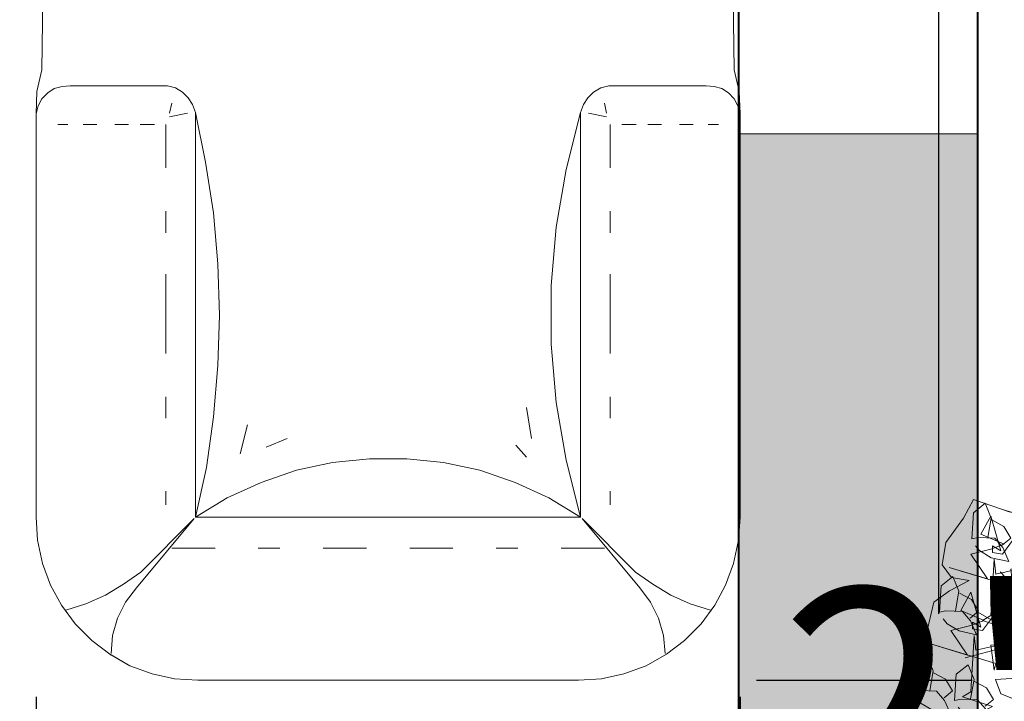
# Model space of a CAD drawing. Units: inches. Extents: x 2337 to 3570, y 1258 to 1938.
# Tile 10 of 30: x 2837 to 2874, y 1626 to 1651. Entities that reach past the tile are written whole.
import ezdxf

# ---------------------------------------------------------------- set-up
doc = ezdxf.new("R2010")
doc.units = ezdxf.units.IN
for name, color, linetype, lineweight in [('A-ANNO-DIMS', 2, 'Continuous', 18), ('A-GLAZ', 4, 'Continuous', 18), ('A-WALL', 7, 'Continuous', 40), ('ARBOL', 74, 'Continuous', 13), ('furn', 8, 'Continuous', 18)]:
    doc.layers.add(name, color=color, linetype=linetype, lineweight=lineweight)
doc.layers.add('A-WALL-PATT', color=18, linetype='Continuous', lineweight=13, true_color=0x000000)
doc.styles.get("Standard").update_dxf_attribs({"font": 'arial.ttf'})
doc.dimstyles.new('ISO-25', dxfattribs={"dimtxt": 9, "dimasz": 2.5, "dimexe": 1.25, "dimexo": 0.625, "dimtad": 1, "dimdec": 1, "dimlunit": 3, "dimtxsty": 'Standard', "dimcen": 2.5, "dimadec": 0, "dimazin": 0, "dimtfac": 1, "dimtdec": 1, "dimtmove": 0, "dimatfit": 3, "dimfxl": 1, "dimarcsym": 0})

# ---------------------------------------------------------------- blocks, each defined once
blk = doc.blocks.new('sofa-49')
at = {"color": 0, "linetype": 'ByBlock'}
for p, q in [((-0.1827, 1.5875), (-0.1944, 0.7614)), ((-0.1827, 1.5875), (-0.1944, 0.7614)), ((0.6696, 0.7614), (0.6579, 1.5875)), ((0.6696, 0.7614), (0.6579, 1.5875)), ((-0.1944, 0.7614), (-0.2007, 0.7344)), ((-0.1944, 0.7614), (-0.2007, 0.7344)), ((0.6759, 0.7344), (0.6696, 0.7614)), ((0.6759, 0.7344), (0.6696, 0.7614)), ((-0.1872, 0.7326), (-0.1791, 0.738)), ((-0.1791, 0.738), (-0.1692, 0.7407)), ((-0.1692, 0.7407), (-0.1593, 0.7416)), ((-0.1593, 0.7416), (-0.0486, 0.7416)), ((-0.0486, 0.7416), (-0.0378, 0.7416)), ((-0.0378, 0.7416), (-0.0279, 0.7389)), ((-0.0279, 0.7389), (-0.0189, 0.7335)), ((0.4941, 0.7335), (0.5031, 0.7389)), ((0.5031, 0.7389), (0.513, 0.7416)), ((0.513, 0.7416), (0.5238, 0.7416)), ((0.5238, 0.7416), (0.6345, 0.7416)), ((0.6345, 0.7416), (0.6444, 0.7407)), ((0.6444, 0.7407), (0.6543, 0.738)), ((0.6543, 0.738), (0.6624, 0.7326)), ((-0.2007, 0.7344), (-0.2016, 0.7065)), ((-0.2007, 0.7344), (-0.2016, 0.7065)), ((-0.1989, 0.7164), (-0.1944, 0.7254)), ((-0.1944, 0.7254), (-0.1872, 0.7326)), ((-0.0189, 0.7335), (-0.0117, 0.7263)), ((-0.0117, 0.7263), (-0.0063, 0.7182)), ((0.4815, 0.7182), (0.4869, 0.7263)), ((0.4869, 0.7263), (0.4941, 0.7335)), ((0.6624, 0.7326), (0.6696, 0.7254)), ((0.6696, 0.7254), (0.6741, 0.7164)), ((0.6768, 0.7065), (0.6759, 0.7344)), ((0.6768, 0.7065), (0.6759, 0.7344)), ((-0.2016, 0.7065), (-0.1989, 0.7164)), ((-0.0351, 0.7074), (-0.0324, 0.72)), ((-0.0063, 0.7182), (-0.0027, 0.7083)), ((0.4779, 0.7083), (0.4815, 0.7182)), ((0.5103, 0.7074), (0.5076, 0.72)), ((0.6741, 0.7164), (0.6768, 0.7065)), ((-0.2016, 0.2034), (-0.2016, 0.7065)), ((-0.2016, 0.7065), (-0.2016, 0.2034)), ((-0.0351, 0.7029), (-0.0126, 0.7074)), ((-0.0027, 0.7083), (-0.0027, 0.6975)), ((0.0099, 0.6462), (-0.0027, 0.7083)), ((0.4779, 0.7083), (0.4599, 0.6372)), ((0.4779, 0.6975), (0.4779, 0.7083)), ((0.5103, 0.7029), (0.4878, 0.7074)), ((0.6768, 0.7065), (0.6768, 0.2034)), ((0.6768, 0.2034), (0.6768, 0.7065)), ((-0.1746, 0.693), (-0.162, 0.693)), ((-0.1431, 0.693), (-0.126, 0.693)), ((-0.1035, 0.693), (-0.0864, 0.693)), ((-0.072, 0.693), (-0.054, 0.693)), ((-0.0396, 0.693), (-0.0396, 0.639)), ((-0.0027, 0.6975), (-0.0027, 0.2034)), ((0.4779, 0.2034), (0.4779, 0.6975)), ((0.5148, 0.693), (0.5148, 0.639)), ((0.5472, 0.693), (0.5292, 0.693)), ((0.5787, 0.693), (0.5616, 0.693)), ((0.6183, 0.693), (0.6012, 0.693)), ((0.6498, 0.693), (0.6372, 0.693)), ((0.0198, 0.5832), (0.0099, 0.6462)), ((0.4599, 0.6372), (0.4473, 0.5652)), ((-0.0396, 0.585), (-0.0396, 0.558)), ((0.0252, 0.5193), (0.0198, 0.5832)), ((0.5148, 0.585), (0.5148, 0.558)), ((0.4473, 0.5652), (0.441, 0.4923)), ((0.027, 0.4554), (0.0252, 0.5193)), ((-0.0396, 0.4077), (-0.0396, 0.5067)), ((0.5148, 0.4077), (0.5148, 0.5067)), ((0.441, 0.4923), (0.441, 0.4194)), ((0.0252, 0.3924), (0.027, 0.4554)), ((0.441, 0.4194), (0.4473, 0.3465)), ((0.0198, 0.3285), (0.0252, 0.3924)), ((-0.0396, 0.3267), (-0.0396, 0.3537)), ((0.4473, 0.3465), (0.4599, 0.2745)), ((0.5148, 0.3267), (0.5148, 0.3537)), ((0.4167, 0.3015), (0.4104, 0.3402)), ((0.0108, 0.2655), (0.0198, 0.3285)), ((0.0531, 0.2826), (0.0621, 0.3186)), ((0.0855, 0.2907), (0.1116, 0.3015)), ((0.4104, 0.2781), (0.3969, 0.2934)), ((0.1683, 0.2718), (0.1233, 0.2619)), ((0.2142, 0.2763), (0.1683, 0.2718)), ((0.261, 0.2763), (0.2142, 0.2763)), ((0.3069, 0.2718), (0.261, 0.2763)), ((0.3519, 0.2619), (0.3069, 0.2718)), ((0.4599, 0.2745), (0.4779, 0.2034)), ((-0.0027, 0.2034), (0.0108, 0.2655)), ((0.1233, 0.2619), (0.0792, 0.2466)), ((0.396, 0.2466), (0.3519, 0.2619)), ((0.0792, 0.2466), (0.0369, 0.2277)), ((0.4383, 0.2277), (0.396, 0.2466)), ((-0.0396, 0.2187), (-0.0396, 0.2358)), ((0.5148, 0.2187), (0.5148, 0.2358)), ((0.0369, 0.2277), (-0.0027, 0.2034)), ((0.4779, 0.2034), (0.4383, 0.2277)), ((-0.1998, 0.1746), (-0.2016, 0.2034)), ((-0.2016, 0.2034), (-0.1998, 0.1746)), ((-0.0765, 0.1152), (-0.0045, 0.2016)), ((-0.0045, 0.2016), (-0.0711, 0.135)), ((-0.0027, 0.2034), (0.2376, 0.2034)), ((0.2376, 0.2034), (0.4779, 0.2034)), ((0.5463, 0.135), (0.4797, 0.2016)), ((0.4797, 0.2016), (0.5517, 0.1152)), ((0.6768, 0.2034), (0.675, 0.1746)), ((0.675, 0.1746), (0.6768, 0.2034)), ((-0.1935, 0.1458), (-0.1998, 0.1746)), ((-0.1998, 0.1746), (-0.1935, 0.1458)), ((0.675, 0.1746), (0.6687, 0.1458)), ((0.6687, 0.1458), (0.675, 0.1746)), ((-0.0324, 0.1647), (0.0216, 0.1647)), ((0.0756, 0.1647), (0.1026, 0.1647)), ((0.1566, 0.1647), (0.2106, 0.1647)), ((0.3186, 0.1647), (0.2646, 0.1647)), ((0.3996, 0.1647), (0.3726, 0.1647)), ((0.5076, 0.1647), (0.4536, 0.1647)), ((-0.1836, 0.1188), (-0.1935, 0.1458)), ((-0.1935, 0.1458), (-0.1836, 0.1188)), ((0.6687, 0.1458), (0.6588, 0.1188)), ((0.6588, 0.1188), (0.6687, 0.1458)), ((-0.0711, 0.135), (-0.0927, 0.1197)), ((0.5679, 0.1197), (0.5463, 0.135)), ((-0.1701, 0.0936), (-0.1836, 0.1188)), ((-0.1836, 0.1188), (-0.1701, 0.0936)), ((-0.0927, 0.1197), (-0.1152, 0.1062)), ((-0.09, 0.0972), (-0.0765, 0.1152)), ((0.5517, 0.1152), (0.5652, 0.0972)), ((0.5904, 0.1062), (0.5679, 0.1197)), ((0.6588, 0.1188), (0.6453, 0.0936)), ((0.6453, 0.0936), (0.6588, 0.1188)), ((-0.1152, 0.1062), (-0.1395, 0.0954)), ((0.6147, 0.0954), (0.5904, 0.1062)), ((-0.153, 0.0702), (-0.1701, 0.0936)), ((-0.1701, 0.0936), (-0.153, 0.0702)), ((-0.1395, 0.0954), (-0.1647, 0.0873)), ((-0.0999, 0.0774), (-0.09, 0.0972)), ((0.5652, 0.0972), (0.5751, 0.0774)), ((0.6399, 0.0873), (0.6147, 0.0954)), ((0.6453, 0.0936), (0.6282, 0.0702)), ((0.6282, 0.0702), (0.6453, 0.0936)), ((-0.1062, 0.0558), (-0.0999, 0.0774)), ((0.5751, 0.0774), (0.5814, 0.0558)), ((-0.1323, 0.0495), (-0.153, 0.0702)), ((-0.153, 0.0702), (-0.1323, 0.0495)), ((0.6282, 0.0702), (0.6075, 0.0495)), ((0.6075, 0.0495), (0.6282, 0.0702)), ((-0.1098, 0.0324), (-0.1323, 0.0495)), ((-0.1323, 0.0495), (-0.1082, 0.0312)), ((-0.108, 0.0333), (-0.1062, 0.0558)), ((0.5814, 0.0558), (0.5832, 0.0333)), ((0.6075, 0.0495), (0.585, 0.0324)), ((0.585, 0.0324), (0.6075, 0.0495)), ((-0.0846, 0.018), (-0.1098, 0.0324)), ((-0.1082, 0.0312), (-0.1081, 0.0315)), ((-0.1081, 0.0315), (-0.0846, 0.018)), ((0.585, 0.0324), (0.5598, 0.018)), ((0.5598, 0.018), (0.585, 0.0324)), ((-0.0567, 0.0081), (-0.0846, 0.018)), ((-0.0846, 0.018), (-0.0567, 0.0081)), ((0.5598, 0.018), (0.5319, 0.0081)), ((0.5319, 0.0081), (0.5598, 0.018)), ((-0.0288, 0.0018), (-0.0567, 0.0081)), ((-0.0567, 0.0081), (-0.0288, 0.0018)), ((0, 0), (-0.0288, 0.0018)), ((-0.0288, 0.0018), (0, 0)), ((0.2376, 0), (0, 0)), ((0, 0), (0.2376, 0)), ((0.4752, 0), (0.2376, 0)), ((0.2376, 0), (0.4752, 0)), ((0.504, 0.0018), (0.4752, 0)), ((0.4752, 0), (0.504, 0.0018)), ((0.5319, 0.0081), (0.504, 0.0018)), ((0.504, 0.0018), (0.5319, 0.0081))]:
    blk.add_line(p, q, dxfattribs=at)
blk = doc.blocks.new('fresno')
at = {"layer": 'ARBOL'}
blk.add_line((-3.638, 1.194), (-4.164, 1.76), dxfattribs=at)
for points in [[(-4.062, 2.379), (-4.443, 2.512), (-4.546, 2.316), (-4.73, 2.062), (-4.767, 1.832), (-4.671, 1.698), (-4.486, 1.667), (-4.693, 1.559), (-4.854, 1.444), (-4.934, 1.102), (-5.037, 0.905), (-5.175, 0.644), (-5.166, 0.406)], [(-3.434, 2.752), (-3.59, 2.546), (-3.693, 2.563), (-3.693, 2.632), (-3.607, 2.58), (-3.71, 2.942), (-3.814, 2.752), (-3.572, 2.649), (-3.71, 2.597), (-3.917, 2.546), (-3.745, 2.287), (-4.142, 2.408), (-3.452, 2.201), (-3.469, 2.132), (-3.503, 2.39), (-3.348, 2.408), (-3.659, 2.339), (-3.676, 2.494), (-3.71, 1.908), (-3.797, 1.856), (-3.486, 1.753), (-3.555, 1.718), (-3.607, 1.666)], [(-4.422, 2.03), (-4.381, 1.979), (-4.257, 1.905), (-4.075, 1.865), (-4.138, 2.012), (-4.221, 2.108), (-4.393, 2.114), (-4.461, 2.101), (-4.444, 2.372), (-4.32, 2.472), (-4.257, 2.318), (-4.293, 2.116)], [(-3.986, 2.149), (-4.142, 1.942), (-4.245, 1.959), (-4.245, 2.028), (-4.159, 1.977), (-4.262, 2.339), (-4.366, 2.149), (-4.124, 2.046), (-4.262, 1.994), (-4.47, 1.942), (-4.297, 1.684), (-4.694, 1.804), (-4.004, 1.597), (-4.021, 1.528), (-4.055, 1.787), (-3.9, 1.804), (-4.211, 1.735), (-4.228, 1.89), (-4.262, 1.304), (-4.349, 1.253), (-4.038, 1.149), (-4.107, 1.115), (-4.159, 1.063)], [(-4.253, 2.298), (-4.127, 2.231), (-4.054, 2.109), (-4.142, 2.039)], [(-4.759, 1.269), (-4.718, 1.217), (-4.593, 1.144), (-4.411, 1.103), (-4.475, 1.25), (-4.557, 1.346), (-4.729, 1.352), (-4.797, 1.339), (-4.78, 1.611), (-4.656, 1.71), (-4.594, 1.557), (-4.629, 1.354)], [(-4.193, 1.356), (-4.349, 1.149), (-4.452, 1.166), (-4.452, 1.235), (-4.366, 1.184), (-4.469, 1.546), (-4.573, 1.356), (-4.331, 1.253), (-4.469, 1.201), (-4.677, 1.149), (-4.504, 0.89), (-4.901, 1.011), (-4.211, 0.804), (-4.228, 0.735), (-4.262, 0.994), (-4.107, 1.011), (-4.418, 0.942), (-4.435, 1.097), (-4.469, 0.511), (-4.556, 0.459), (-4.245, 0.356), (-4.314, 0.322), (-4.366, 0.27)], [(-4.589, 1.536), (-4.464, 1.469), (-4.391, 1.348), (-4.478, 1.277)], [(-3.192, 1.017), (-3.578, 1.215), (-3.949, 1.081), (-4.398, 1.339)], [(-3.354, 1.176), (-4.529, 0.864)], [(-5.028, 0.44), (-4.987, 0.388), (-4.862, 0.315), (-4.68, 0.274), (-4.744, 0.421), (-4.826, 0.517), (-4.998, 0.523), (-5.066, 0.511), (-5.049, 0.782), (-4.925, 0.881), (-4.863, 0.728), (-4.898, 0.525)], [(-4.602, 0.35), (-4.561, 0.299), (-4.436, 0.225), (-4.254, 0.185), (-4.318, 0.332), (-4.4, 0.428), (-4.572, 0.433), (-4.64, 0.421), (-4.623, 0.692), (-4.499, 0.792), (-4.437, 0.638), (-4.472, 0.436)], [(-4.858, 0.707), (-4.733, 0.64), (-4.66, 0.519), (-4.747, 0.448)], [(-4.432, 0.618), (-4.307, 0.55), (-4.234, 0.429), (-4.321, 0.359)], [(-3.824, 0.404), (-3.763, 0.427), (-3.654, 0.523), (-3.559, 0.683), (-3.719, 0.668), (-3.835, 0.62), (-3.894, 0.457), (-3.903, 0.389), (-4.156, 0.489), (-4.212, 0.638), (-4.047, 0.65), (-3.865, 0.553)]]:
    blk.add_lwpolyline(points, dxfattribs=at)
blk = doc.blocks.new('*D86')
at = {"layer": 'A-ANNO-DIMS', "color": 0, "lineweight": -2, "transparency": 16777216}
for p, q in [((2762.092, 1679.329), (2762.092, 1663.443)), ((2863.836, 1679.329), (2863.836, 1663.443)), ((2762.092, 1664.693), (2617.848, 1664.693)), ((2861.336, 1664.693), (2764.592, 1664.693))]:
    blk.add_line(p, q, dxfattribs=at)
at = {"layer": 'A-ANNO-DIMS', "color": 0, "transparency": 16777216}
for points in [[(2764.592, 1665.109), (2764.592, 1664.276), (2762.092, 1664.693)], [(2861.336, 1665.109), (2861.336, 1664.276), (2863.836, 1664.693)]]:
    blk.add_solid(points, dxfattribs=at)
at = {"layer": 'Defpoints', "color": 0, "transparency": 16777216}
for p in [(2762.092, 1679.954), (2863.836, 1679.954), (2762.092, 1664.693)]:
    blk.add_point(p, dxfattribs=at)
at = {"layer": 'A-ANNO-DIMS', "color": 0, "transparency": 16777216, "insert": (2688.72, 1669.974), "char_height": 9, "attachment_point": 5}
blk.add_mtext('CORNER SOFA 8\'-5 1/2"', dxfattribs=at)
blk = doc.blocks.new('*D90')
at = {"layer": 'A-ANNO-DIMS', "color": 0, "lineweight": -2, "transparency": 16777216}
for p, q in [((2871.382, 1676.497), (2871.382, 1796.695)), ((2864.515, 1676.497), (2872.632, 1676.497)), ((2871.382, 1629.048), (2871.382, 1673.997)), ((2864.515, 1626.548), (2872.632, 1626.548))]:
    blk.add_line(p, q, dxfattribs=at)
at = {"layer": 'A-ANNO-DIMS', "color": 0, "transparency": 16777216}
for points in [[(2870.966, 1673.997), (2871.799, 1673.997), (2871.382, 1676.497)], [(2870.966, 1629.048), (2871.799, 1629.048), (2871.382, 1626.548)]]:
    blk.add_solid(points, dxfattribs=at)
at = {"layer": 'Defpoints', "color": 0, "transparency": 16777216}
for p in [(2863.89, 1676.497), (2871.382, 1676.497), (2863.89, 1626.548)]:
    blk.add_point(p, dxfattribs=at)
at = {"layer": 'A-ANNO-DIMS', "color": 0, "transparency": 16777216, "insert": (2866.101, 1737.846), "char_height": 9, "attachment_point": 5, "rotation": 90}
blk.add_mtext('LOUNGE SEAT 4\'-2"', dxfattribs=at)
blk = doc.blocks.new('*D91')
at = {"layer": 'A-ANNO-DIMS', "color": 0, "lineweight": -2, "transparency": 16777216}
for p, q in [((2837.379, 1625.923), (2837.379, 1617.806)), ((2863.89, 1625.923), (2863.89, 1617.806)), ((2839.879, 1619.056), (2861.39, 1619.056)), ((2863.89, 1619.056), (2912.689, 1619.056))]:
    blk.add_line(p, q, dxfattribs=at)
at = {"layer": 'A-ANNO-DIMS', "color": 0, "transparency": 16777216}
for points in [[(2839.879, 1619.473), (2839.879, 1618.639), (2837.379, 1619.056)], [(2861.39, 1619.473), (2861.39, 1618.639), (2863.89, 1619.056)]]:
    blk.add_solid(points, dxfattribs=at)
at = {"layer": 'Defpoints', "color": 0, "transparency": 16777216}
for p in [(2837.379, 1626.548), (2863.89, 1626.548), (2863.89, 1619.056)]:
    blk.add_point(p, dxfattribs=at)
at = {"layer": 'A-ANNO-DIMS', "color": 0, "transparency": 16777216, "insert": (2889.54, 1624.335), "char_height": 9, "attachment_point": 5}
blk.add_mtext('2\'-2 1/2"', dxfattribs=at)

msp = doc.modelspace()

# ---------------------------------------------------------------- hatches: boundary and pattern name
at = {"layer": 'A-WALL-PATT'}
h = msp.add_hatch(color=256, dxfattribs=at)
h.dxf.hatch_style = 1
h.paths.add_polyline_path([(2671.836, 1857.116), (2455.836, 1857.116), (2455.836, 1824.116), (2464.836, 1824.116), (2464.836, 1848.116), (2671.836, 1848.116)])
h.paths.add_polyline_path([(2566.836, 1764.116), (2464.836, 1764.116), (2464.836, 1788.116), (2455.836, 1788.116), (2455.836, 1743.116), (2464.836, 1743.116), (2464.836, 1755.116), (2566.836, 1755.116)])
h.paths.add_polyline_path([(2683.836, 1761.116), (2683.836, 1764.116), (2602.836, 1764.116), (2602.836, 1755.116), (2608.836, 1755.116), (2608.836, 1701.116), (2662.836, 1701.116), (2662.836, 1605.116), (2671.836, 1605.116), (2671.836, 1713.116), (2662.836, 1713.116), (2662.836, 1707.116), (2614.836, 1707.116), (2614.836, 1755.116), (2662.836, 1755.116), (2662.836, 1749.116), (2671.836, 1749.116), (2671.836, 1755.116), (2683.836, 1755.116)])
h.paths.add_polyline_path([(2464.836, 1707.116), (2455.836, 1707.116), (2455.836, 1617.116), (2464.836, 1617.116), (2464.836, 1635.116), (2506.836, 1635.116), (2506.836, 1641.116), (2464.836, 1641.116)])
h.paths.add_polyline_path([(2542.836, 1551.116), (2464.836, 1551.116), (2464.836, 1569.116), (2455.836, 1569.116), (2455.836, 1518.116), (2464.836, 1518.116), (2464.836, 1542.116), (2542.836, 1542.116)])
h.paths.add_polyline_path([(2464.836, 1482.116), (2455.836, 1482.116), (2455.836, 1410.116), (2464.836, 1410.116)])
h.paths.add_polyline_path([(2626.836, 1350.116), (2590.836, 1350.116), (2590.836, 1380.116), (2584.836, 1380.116), (2584.836, 1350.116), (2464.836, 1350.116), (2464.836, 1374.116), (2455.836, 1374.116), (2455.836, 1341.116), (2626.836, 1341.116)])
h.paths.add_polyline_path([(2662.836, 1416.116), (2686.836, 1416.116), (2686.836, 1422.116), (2590.836, 1422.116), (2590.836, 1542.116), (2680.836, 1542.116), (2680.836, 1551.116), (2671.836, 1551.116), (2671.836, 1557.116), (2662.836, 1557.116), (2662.836, 1551.116), (2578.836, 1551.116), (2578.836, 1542.116), (2584.836, 1542.116), (2584.836, 1410.116), (2590.836, 1410.116), (2590.836, 1416.116), (2656.836, 1416.116), (2656.836, 1350.116), (2650.836, 1350.116), (2650.836, 1341.116), (2731.836, 1341.116), (2731.836, 1362.116), (2722.836, 1362.116), (2722.836, 1350.116), (2662.836, 1350.116)])
h.paths.add_polyline_path([(2731.836, 1434.116), (2722.836, 1434.116), (2722.836, 1422.116), (2716.836, 1422.116), (2716.836, 1416.116), (2722.836, 1416.116), (2722.836, 1386.116), (2731.836, 1386.116)], flags=17)
h.paths.add_polyline_path([(2731.836, 1542.116), (2752.836, 1542.116), (2752.836, 1551.116), (2716.836, 1551.116), (2716.836, 1545.116), (2716.836, 1542.116), (2722.836, 1542.116), (2722.836, 1482.116), (2731.836, 1482.116)])
h.paths.add_polyline_path([(2809.836, 1551.116), (2788.836, 1551.116), (2788.836, 1542.116), (2809.836, 1542.116), (2809.836, 1548.116)])
h.paths.add_polyline_path([(2872.836, 1647.116), (2863.836, 1647.116), (2863.836, 1551.116), (2857.836, 1551.116), (2857.836, 1548.116), (2857.836, 1542.116), (2872.836, 1542.116)])
h.paths.add_polyline_path([(2872.836, 1764.116), (2827.836, 1764.116), (2827.836, 1755.116), (2863.836, 1755.116), (2863.836, 1719.116), (2872.836, 1719.116)])
h.paths.add_polyline_path([(2755.836, 1764.116), (2719.836, 1764.116), (2719.836, 1755.116), (2755.836, 1755.116)])

# ---------------------------------------------------------------- linework, layer by layer
at = {"layer": 'A-GLAZ'}
msp.add_line((2872.836, 1647.116), (2863.836, 1647.116), dxfattribs=at)
at = {"layer": 'A-WALL'}
for p, q in [((2872.836, 1764.116), (2872.836, 1542.116)), ((2863.836, 1755.116), (2863.836, 1551.116))]:
    msp.add_line(p, q, dxfattribs=at)

# ---------------------------------------------------------------- block references
at = {"layer": 'ARBOL', "xscale": 3.617267037020409, "yscale": 3.617267037020409, "zscale": 3.617267037020409}
msp.add_blockref('fresno', (2888.753, 1624.269), dxfattribs=at)
at = {"layer": 'furn', "xscale": 30.18064521598093, "yscale": 30.18064521598093, "zscale": 30.18064521598093}
msp.add_blockref('sofa-49', (2843.464, 1626.548), dxfattribs=at)

# ---------------------------------------------------------------- dimensions: what is measured, and where the dimension line sits
at = {"layer": 'A-ANNO-DIMS'}
for base, p1, p2, angle, text, picture, middle in [((2871.382, 1676.497), (2863.89, 1626.548), (2863.89, 1676.497), 90, 'LOUNGE SEAT <>', '*D90', (2866.101, 1737.846)), ((2762.092, 1664.693), (2863.836, 1679.954), (2762.092, 1679.954), 180, 'CORNER SOFA <>', '*D86', (2688.72, 1669.974))]:
    dim = msp.add_linear_dim(base=base, p1=p1, p2=p2, angle=angle, text=text, dimstyle='ISO-25', override={"dimdec": 1, "dimlfac": 1, "dimrnd": 0, "dimzin": 1, "dimdsep": 46, "dimlunit": 4, "dimfrac": 2}, dxfattribs=at)
    dim.commit()
    dim.dimension.update_dxf_attribs({"geometry": picture, "text_midpoint": middle})
dim = msp.add_linear_dim(base=(2863.89, 1619.056), p1=(2837.379, 1626.548), p2=(2863.89, 1626.548), dimstyle='ISO-25', override={"dimdec": 1, "dimlfac": 1, "dimrnd": 0, "dimzin": 1, "dimdsep": 46, "dimlunit": 4, "dimfrac": 2}, dxfattribs=at)
dim.commit()
dim.dimension.update_dxf_attribs({"geometry": '*D91', "text_midpoint": (2889.54, 1624.335)})

doc.saveas('drawing.dxf')
